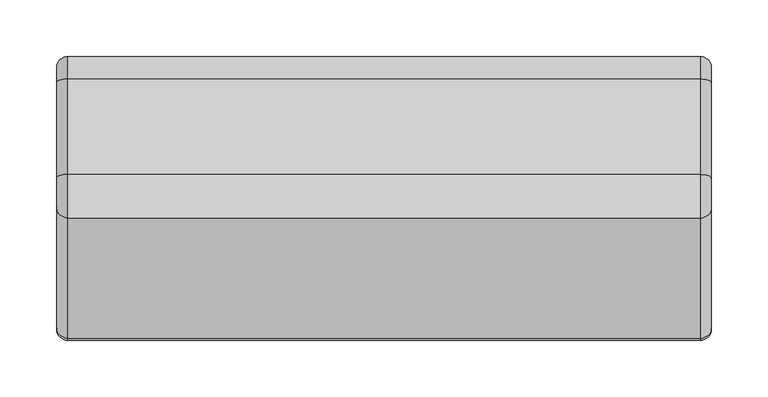
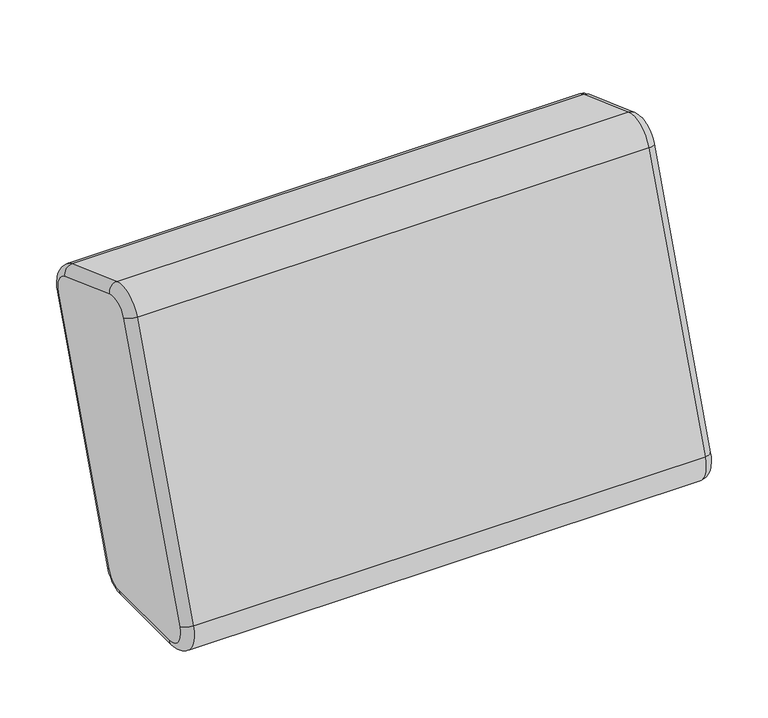
"""IFC4 building model written with IfcOpenShell, lengths in millimetres: furniture geometry."""

from ifc_helpers import new_model, si_unit, point, frame, origin, place, context, project, spatial, circle_curve, ellipse_curve, trimmed, source, transform, mapped, element, save
from ifc_brep_helpers import plane_surface, cylinder_surface, revolved_surface, advanced_brep


def furniture_57072a26(model_context):
    return source(origin(), model_context, "Body", "AdvancedBrep", [
        advanced_brep(
        [(288.5853906, 609.5185405, 469.9348489), (288.5853906, 628.3736149, 483.1373142), (288.5853906, 723.5847628, 744.7277933), (288.5853906, 711.5923743, 770.4455535), (288.5853906, 627.0200384, 801.2273664), (288.5853906, 601.3022782, 789.2349779), (288.5853906, 494.8874666, 496.8626858), (288.5853906, 513.742541, 469.9348489), (-290.0, 513.742541, 469.9348489), (-290.0, 494.8874666, 496.8626858), (-290.0, 601.3022782, 789.2349779), (-290.0, 627.0200384, 801.2273664), (-290.0, 711.5923743, 770.4455535), (-290.0, 723.5847628, 744.7277933), (-290.0, 628.3736149, 483.1373142), (-290.0, 609.5185405, 469.9348489), (-280.0, 630.4402399, 810.6242926), (-280.0, 591.905352, 792.6551793), (278.5854032, 591.905352, 792.6551793), (278.5853906, 630.4402399, 810.6242926), (-280.0, 485.4905403, 500.2828873), (278.5853906, 485.4905403, 500.2828873), (-280.0, 513.742541, 459.9348489), (278.5854029, 513.742541, 459.9348489), (-280.0, 609.5185405, 459.9348489), (278.5854031, 609.5185405, 459.9348489), (-280.0, 637.7705411, 479.7171127), (278.5854031, 637.7705411, 479.7171127), (-280.0, 732.9816891, 741.3075918), (278.5853906, 732.9816891, 741.3075918), (-280.0, 715.0125757, 779.8424797), (278.5854031, 715.0125757, 779.8424797)],
        [
            (0, 1, circle_curve(frame((288.5853906, 609.5185405, 490.0), z_axis=(1.0, 0.0, 0.0), x_axis=(0.0, 0.0, -1.0)), 20.0651511)),
            (1, 2),
            (2, 3, circle_curve(frame((288.5853906, 704.7296884, 751.5904791), z_axis=(1.0, 0.0, 0.0), x_axis=(0.0, 0.9396926207859067, -0.3420201433256736)), 20.0651511)),
            (3, 4),
            (4, 5, circle_curve(frame((288.5853906, 620.1573526, 782.372292), z_axis=(1.0, 0.0, 0.0), x_axis=(0.0, 0.34202014332566927, 0.9396926207859082)), 20.0651511)),
            (5, 6),
            (6, 7, circle_curve(frame((288.5853906, 513.742541, 490.0), z_axis=(1.0, 0.0, 0.0), x_axis=(0.0, -0.939692620785912, 0.3420201433256589)), 20.0651511)),
            (7, 0),
            (8, 9, circle_curve(frame((-290.0, 513.742541, 490.0), z_axis=(-1.0, 0.0, 0.0), x_axis=(0.0, 0.0, -1.0)), 20.0651511)),
            (9, 10),
            (10, 11, circle_curve(frame((-290.0, 620.1573526, 782.372292), z_axis=(-1.0, 0.0, 0.0), x_axis=(0.0, -0.9396926207859104, 0.3420201433256632)), 20.0651511)),
            (11, 12),
            (12, 13, circle_curve(frame((-290.0, 704.7296884, 751.5904791), z_axis=(-1.0, 0.0, 0.0), x_axis=(0.0, 0.34202014332567177, 0.9396926207859073)), 20.0651511)),
            (13, 14),
            (14, 15, circle_curve(frame((-290.0, 609.5185405, 490.0), z_axis=(-1.0, 0.0, 0.0), x_axis=(0.0, 0.9396926207859085, -0.3420201433256683)), 20.0651511)),
            (15, 8),
            (16, 17, circle_curve(frame((-280.0, 620.1573526, 782.372292), z_axis=(1.0, 0.0, 0.0), x_axis=(0.0, 1.0, 0.0)), 30.0651511)),
            (17, 18),
            (18, 19, circle_curve(frame((278.5853906, 620.1573526, 782.372292), z_axis=(-1.0, 0.0, 0.0), x_axis=(0.0, 1.0, 0.0)), 30.0651511)),
            (19, 16),
            (17, 20),
            (20, 21),
            (21, 18),
            (20, 22, circle_curve(frame((-280.0, 513.742541, 490.0), z_axis=(1.0, 0.0, 0.0), x_axis=(0.0, 1.0, 0.0)), 30.0651511)),
            (22, 23),
            (23, 21, circle_curve(frame((278.5853906, 513.742541, 490.0), z_axis=(-1.0, 0.0, 0.0), x_axis=(0.0, 1.0, 0.0)), 30.0651511)),
            (22, 24),
            (24, 25),
            (25, 23),
            (24, 26, circle_curve(frame((-280.0, 609.5185405, 490.0), z_axis=(1.0, 0.0, 0.0), x_axis=(0.0, 1.0, 0.0)), 30.0651511)),
            (26, 27),
            (27, 25, circle_curve(frame((278.5853906, 609.5185405, 490.0), z_axis=(-1.0, 0.0, 0.0), x_axis=(0.0, 1.0, 0.0)), 30.0651511)),
            (26, 28),
            (28, 29),
            (29, 27),
            (28, 30, circle_curve(frame((-280.0, 704.7296884, 751.5904791), z_axis=(1.0, 0.0, 0.0), x_axis=(0.0, 1.0, 0.0)), 30.0651511)),
            (30, 31),
            (31, 29, circle_curve(frame((278.5853906, 704.7296884, 751.5904791), z_axis=(-1.0, 0.0, 0.0), x_axis=(0.0, 1.0, 0.0)), 30.0651511)),
            (30, 16),
            (19, 31),
            (20, 9, circle_curve(frame((-280.0, 494.8874666, 496.8626858), z_axis=(0.0, -0.3420201433256627, -0.9396926207859105), x_axis=(-1.0, 0.0, 0.0)), 10.0)),
            (8, 22, circle_curve(frame((-280.0, 513.742541, 469.9348489), z_axis=(0.0, -1.0, 0.0), x_axis=(-1.0, 0.0, 0.0)), 10.0)),
            (17, 10, circle_curve(frame((-280.0, 601.3022782, 789.2349779), z_axis=(0.0, -0.3420201433256581, -0.9396926207859123), x_axis=(-1.0, 0.0, 0.0)), 10.0)),
            (16, 11, circle_curve(frame((-280.0, 627.0200384, 801.2273664), z_axis=(0.0, -0.9396926207859091, 0.3420201433256669), x_axis=(-1.0, 0.0, 0.0)), 10.0)),
            (30, 12, circle_curve(frame((-280.0, 711.5923743, 770.4455535), z_axis=(0.0, -0.9396926207859227, 0.34202014332562924), x_axis=(-1.0, 0.0, 0.0)), 10.0)),
            (28, 13, circle_curve(frame((-280.0, 723.5847628, 744.7277933), z_axis=(0.0, 0.34202014332566905, 0.9396926207859083), x_axis=(-1.0, 0.0, 0.0)), 10.0)),
            (26, 14, circle_curve(frame((-280.0, 628.3736149, 483.1373142), z_axis=(0.0, 0.3420201433256558, 0.9396926207859131), x_axis=(-1.0, 0.0, 0.0)), 10.0)),
            (24, 15, circle_curve(frame((-280.0, 609.5185405, 469.9348489), z_axis=(0.0, 0.9999999999999999, 0.0), x_axis=(-1.0, 0.0, 0.0)), 10.0)),
            (27, 1, circle_curve(frame((278.5853906, 628.3736149, 483.1373142), z_axis=(0.0, -0.34202014332566655, -0.9396926207859092), x_axis=(1.0, 0.0, 0.0)), 10.0)),
            (0, 25, circle_curve(frame((278.5853906, 609.5185405, 469.9348489), z_axis=(0.0, 1.0, 0.0), x_axis=(1.0, 0.0, 0.0)), 10.0)),
            (29, 2, circle_curve(frame((278.5853906, 723.5847628, 744.7277933), z_axis=(0.0, -0.3420201433256561, -0.939692620785913), x_axis=(1.0, 0.0, 0.0)), 10.0)),
            (31, 3, circle_curve(frame((278.5853906, 711.5923743, 770.4455535), z_axis=(0.0, 0.9396926207859077, -0.3420201433256707), x_axis=(1.0, 0.0, 0.0)), 10.0)),
            (19, 4, circle_curve(frame((278.5853906, 627.0200384, 801.2273664), z_axis=(0.0, 0.9396926207859227, -0.3420201433256294), x_axis=(1.0, 0.0, 0.0)), 10.0)),
            (18, 5, circle_curve(frame((278.5853906, 601.3022782, 789.2349779), z_axis=(0.0, 0.34202014332566893, 0.9396926207859083), x_axis=(1.0, 0.0, 0.0)), 10.0)),
            (21, 6, circle_curve(frame((278.5853906, 494.8874666, 496.8626858), z_axis=(0.0, 0.3420201433256583, 0.9396926207859122), x_axis=(1.0, 0.0, 0.0)), 10.0)),
            (23, 7, circle_curve(frame((278.5853906, 513.742541, 469.9348489), z_axis=(0.0, -1.0, 0.0), x_axis=(1.0, 0.0, 0.0)), 10.0)),
        ],
        [
            plane_surface(frame((288.5853906, 650.2225036, 782.372292), z_axis=(1.0, 0.0, 0.0), x_axis=(0.0, 0.0, 1.0))),
            plane_surface(frame((-290.0, 650.2225036, 782.372292), z_axis=(-1.0, 0.0, 0.0), x_axis=(0.0, 0.0, -1.0))),
            cylinder_surface(frame((-290.0, 620.1573526, 782.372292), z_axis=(1.0, 0.0, 0.0), x_axis=(0.0, 1.0, 0.0)), 30.0651511),
            plane_surface(frame((288.5853906, 591.905352, 792.6551793), z_axis=(0.0, -0.9396926207859123, 0.3420201433256582), x_axis=(-1.0, 0.0, 0.0))),
            cylinder_surface(frame((-290.0, 513.742541, 490.0), z_axis=(1.0, 0.0, 0.0), x_axis=(0.0, 1.0, 0.0)), 30.0651511),
            plane_surface(frame((288.5853906, 513.742541, 459.9348489), z_axis=(0.0, 0.0, -1.0), x_axis=(-1.0, 0.0, 0.0))),
            cylinder_surface(frame((-290.0, 609.5185405, 490.0), z_axis=(1.0, 0.0, 0.0), x_axis=(0.0, 1.0, 0.0)), 30.0651511),
            plane_surface(frame((288.5853906, 637.7705411, 479.7171127), z_axis=(0.0, 0.9396926207859131, -0.3420201433256561), x_axis=(-1.0, 0.0, 0.0))),
            cylinder_surface(frame((-290.0, 704.7296884, 751.5904791), z_axis=(1.0, 0.0, 0.0), x_axis=(0.0, 1.0, 0.0)), 30.0651511),
            plane_surface(frame((288.5853906, 715.0125757, 779.8424797), z_axis=(0.0, 0.34202014332562936, 0.9396926207859227), x_axis=(-1.0, 0.0, 0.0))),
            revolved_surface(trimmed(ellipse_curve(frame((-280.0, 513.742541, 469.9348489), z_axis=(0.0, 1.0, 0.0), x_axis=(-1.0, 0.0, 0.0)), 10.0, 10.0), [point((-280.0, 513.742541, 459.9348489))], [point((-290.0, 513.742541, 469.9348489))], True, "CARTESIAN"), (-290.0, 513.742541, 490.0), (-1.0, 0.0, 0.0)),
            cylinder_surface(frame((-280.0, 494.8874666, 496.8626858), z_axis=(0.0, 0.3420201433256581, 0.9396926207859123), x_axis=(-1.0, 0.0, 0.0)), 10.0),
            revolved_surface(trimmed(ellipse_curve(frame((-280.0, 601.3022782, 789.2349779), z_axis=(0.0, -0.34202014332566316, -0.9396926207859104), x_axis=(-1.0, 0.0, 0.0)), 10.0, 10.0), [point((-280.0, 591.905352, 792.6551793))], [point((-290.0, 601.3022782, 789.2349779))], True, "CARTESIAN"), (-290.0, 620.1573526, 782.372292), (-1.0, 0.0, 0.0)),
            cylinder_surface(frame((-280.0, 627.0200384, 801.2273664), z_axis=(0.0, 0.9396926207859227, -0.34202014332562924), x_axis=(-1.0, 0.0, 0.0)), 10.0),
            revolved_surface(trimmed(ellipse_curve(frame((-280.0, 711.5923743, 770.4455535), z_axis=(0.0, -0.9396926207859074, 0.3420201433256716), x_axis=(-1.0, 0.0, 0.0)), 10.0, 10.0), [point((-280.0, 715.0125757, 779.8424797))], [point((-290.0, 711.5923743, 770.4455535))], True, "CARTESIAN"), (-290.0, 704.7296884, 751.5904791), (-1.0, 0.0, 0.0)),
            cylinder_surface(frame((-280.0, 723.5847628, 744.7277933), z_axis=(0.0, -0.3420201433256558, -0.9396926207859131), x_axis=(-1.0, 0.0, 0.0)), 10.0),
            revolved_surface(trimmed(ellipse_curve(frame((-280.0, 628.3736149, 483.1373142), z_axis=(0.0, 0.34202014332566805, 0.9396926207859086), x_axis=(-1.0, 0.0, 0.0)), 10.0, 10.0), [point((-280.0, 637.7705411, 479.7171127))], [point((-290.0, 628.3736149, 483.1373142))], True, "CARTESIAN"), (-290.0, 609.5185405, 490.0), (-1.0, 0.0, 0.0)),
            cylinder_surface(frame((-280.0, 609.5185405, 469.9348489), z_axis=(0.0, -1.0, 0.0), x_axis=(-1.0, 0.0, 0.0)), 10.0),
            revolved_surface(trimmed(ellipse_curve(frame((278.5853906, 609.5185405, 469.9348489), z_axis=(0.0, -1.0, 0.0), x_axis=(1.0, 0.0, 0.0)), 10.0, 10.0), [point((278.5853906, 609.5185405, 459.9348489))], [point((288.5853906, 609.5185405, 469.9348489))], True, "CARTESIAN"), (288.5853906, 609.5185405, 490.0), (1.0, 0.0, 0.0)),
            cylinder_surface(frame((278.5853906, 628.3736149, 483.1373142), z_axis=(0.0, 0.3420201433256561, 0.939692620785913), x_axis=(1.0, 0.0, 0.0)), 10.0),
            revolved_surface(trimmed(ellipse_curve(frame((278.5853906, 723.5847628, 744.7277933), z_axis=(0.0, -0.3420201433256738, -0.9396926207859065), x_axis=(1.0, 0.0, 0.0)), 10.0, 10.0), [point((278.5853906, 732.9816891, 741.3075918))], [point((288.5853906, 723.5847628, 744.7277933))], True, "CARTESIAN"), (288.5853906, 704.7296884, 751.5904791), (1.0, 0.0, 0.0)),
            cylinder_surface(frame((278.5853906, 711.5923743, 770.4455535), z_axis=(0.0, -0.9396926207859227, 0.3420201433256294), x_axis=(1.0, 0.0, 0.0)), 10.0),
            revolved_surface(trimmed(ellipse_curve(frame((278.5853906, 627.0200384, 801.2273664), z_axis=(0.0, 0.9396926207859082, -0.3420201433256693), x_axis=(1.0, 0.0, 0.0)), 10.0, 10.0), [point((278.5853906, 630.4402399, 810.6242926))], [point((288.5853906, 627.0200384, 801.2273664))], True, "CARTESIAN"), (288.5853906, 620.1573526, 782.372292), (1.0, 0.0, 0.0)),
            cylinder_surface(frame((278.5853906, 601.3022782, 789.2349779), z_axis=(0.0, -0.3420201433256583, -0.9396926207859122), x_axis=(1.0, 0.0, 0.0)), 10.0),
            revolved_surface(trimmed(ellipse_curve(frame((278.5853906, 494.8874666, 496.8626858), z_axis=(0.0, 0.34202014332565894, 0.939692620785912), x_axis=(1.0, 0.0, 0.0)), 10.0, 10.0), [point((278.5853906, 485.4905403, 500.2828873))], [point((288.5853906, 494.8874666, 496.8626858))], True, "CARTESIAN"), (288.5853906, 513.742541, 490.0), (1.0, 0.0, 0.0)),
            cylinder_surface(frame((278.5853906, 513.742541, 469.9348489), z_axis=(0.0, 1.0, 0.0), x_axis=(1.0, 0.0, 0.0)), 10.0),
        ],
        [
            (0, [[1, 2, 3, 4, 5, 6, 7, 8]]),
            (1, [[9, 10, 11, 12, 13, 14, 15, 16]]),
            (2, [[17, 18, 19, 20]]),
            (3, [[21, 22, 23, -18]]),
            (4, [[24, 25, 26, -22]]),
            (5, [[27, 28, 29, -25]]),
            (6, [[30, 31, 32, -28]]),
            (7, [[33, 34, 35, -31]]),
            (8, [[36, 37, 38, -34]]),
            (9, [[39, -20, 40, -37]]),
            (10, [[41, -9, 42, -24]]),
            (11, [[-41, -21, 43, -10]]),
            (12, [[-43, -17, 44, -11]]),
            (13, [[-44, -39, 45, -12]]),
            (14, [[-45, -36, 46, -13]]),
            (15, [[-46, -33, 47, -14]]),
            (16, [[-47, -30, 48, -15]]),
            (17, [[-42, -16, -48, -27]]),
            (18, [[49, -1, 50, -32]]),
            (19, [[-49, -35, 51, -2]]),
            (20, [[-51, -38, 52, -3]]),
            (21, [[-52, -40, 53, -4]]),
            (22, [[-53, -19, 54, -5]]),
            (23, [[-54, -23, 55, -6]]),
            (24, [[-55, -26, 56, -7]]),
            (25, [[-50, -8, -56, -29]]),
        ],
    ),
    ])


if __name__ == "__main__":
    model = new_model("IFC4")
    model_context = context("Model", 3, world=origin())
    ifc_project = project(units=[si_unit("LENGTHUNIT", "METRE", prefix="MILLI")], contexts=[model_context])
    site = spatial("IfcSite", under=ifc_project)
    building = spatial("IfcBuilding", under=site)
    placement = place(None, origin())
    furniture_shape = furniture_57072a26(model_context)
    element("IfcFurniture", 1, at=placement, inside=building, context=model_context, shape_type="MappedRepresentation", body=[
        mapped(furniture_shape, transform((0.0, 0.0, 0.0), x_axis=(1.0, 0.0, 0.0), y_axis=(0.0, 1.0, 0.0), z_axis=(0.0, 0.0, 1.0))),
    ])
    save(model, "model.ifc")

# Revit data of these elements
# Type
#   Width [instance] = 6' - 3.19685"
#   Default Elevation = 0
